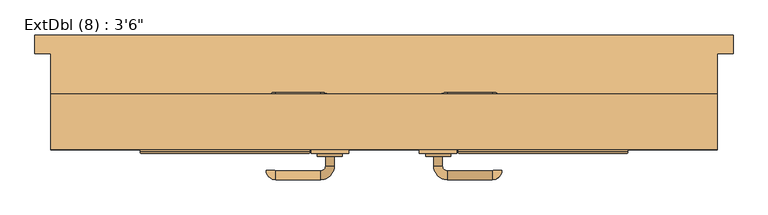
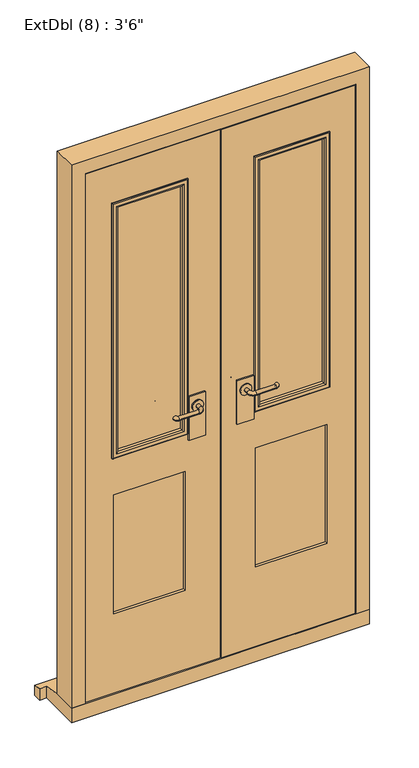
"""IFC4 building model written with IfcOpenShell, lengths in millimetres: door geometry."""

from ifc_helpers import new_model, si_unit, point, frame, frame_2d, origin, place, context, project, spatial, polyline, circle_curve, ellipse_curve, trimmed, segment, composite_curve, outline, extrude, faceted_brep, source, transform, mapped, element, save
from ifc_brep_helpers import plane_surface, cylinder_surface, revolved_surface, advanced_brep


def door_2576ec39(model_context):
    return source(origin(), model_context, "Body", "SolidModel", [
        extrude(outline(composite_curve([segment(trimmed(circle_curve(frame_2d((1050.0, 86.5)), 20.0), [point((1050.0, 66.5))], [point((1050.0, 106.5))], False, "CARTESIAN"), True, "CONTINUOUS"), segment(trimmed(circle_curve(frame_2d((1050.0, 86.5)), 20.0), [point((1050.0, 106.5))], [point((1050.0, 66.5))], False, "CARTESIAN"), True, "CONTINUOUS")], self_intersect=False)), frame((0.0, -88.3929895, 0.0), z_axis=(0.0, 1.0, 0.0), x_axis=(0.0, 0.0, 1.0)), (0.0, 0.0, 1.0), 4.5929895),
        advanced_brep(
        [(93.5, -88.3929895, 1050.0), (79.5, -88.3929895, 1050.0), (79.5, -103.8, 1050.0), (93.5, -103.8, 1050.0), (101.5, -125.8, 1050.0), (101.5, -111.8, 1050.0), (173.5, -125.8, 1050.0), (173.5, -111.8, 1050.0), (174.5, -110.8, 1050.0), (188.5, -110.8, 1050.0)],
        [
            (0, 1, circle_curve(frame((86.5, -88.3929895, 1050.0), z_axis=(0.0, 1.0, 0.0), x_axis=(-1.0, 0.0, 0.0)), 7.0)),
            (1, 0, circle_curve(frame((86.5, -88.3929895, 1050.0), z_axis=(0.0, 1.0, 0.0), x_axis=(-1.0, 0.0, 0.0)), 7.0)),
            (1, 2),
            (2, 3, circle_curve(frame((86.5, -103.8, 1050.0), z_axis=(0.0, 1.0, 0.0), x_axis=(-1.0, 0.0, 0.0)), 7.0)),
            (3, 0),
            (3, 2, circle_curve(frame((86.5, -103.8, 1050.0), z_axis=(0.0, 1.0, 0.0), x_axis=(-1.0, 0.0, 0.0)), 7.0)),
            (4, 5, circle_curve(frame((101.5, -118.8, 1050.0), z_axis=(-1.0, 0.0, 0.0), x_axis=(0.0, -1.0, 0.0)), 7.0)),
            (5, 3, circle_curve(frame((101.5, -103.8, 1050.0), z_axis=(0.0, 0.0, -1.0), x_axis=(-1.0, 0.0, 0.0)), 8.0)),
            (2, 4, circle_curve(frame((101.5, -103.8, 1050.0), z_axis=(0.0, 0.0, 1.0), x_axis=(-1.0, 0.0, 0.0)), 22.0)),
            (5, 4, circle_curve(frame((101.5, -118.8, 1050.0), z_axis=(-1.0, 0.0, 0.0), x_axis=(0.0, -1.0, 0.0)), 7.0)),
            (4, 6),
            (6, 7, circle_curve(frame((173.5, -118.8, 1050.0), z_axis=(-1.0, 0.0, 0.0), x_axis=(0.0, -1.0, 0.0)), 7.0)),
            (7, 5),
            (7, 6, circle_curve(frame((173.5, -118.8, 1050.0), z_axis=(-1.0, 0.0, 0.0), x_axis=(0.0, -1.0, 0.0)), 7.0)),
            (8, 9, circle_curve(frame((181.5, -110.8, 1050.0), z_axis=(0.0, 1.0, 0.0), x_axis=(1.0, 0.0, 0.0)), 7.0)),
            (9, 8, circle_curve(frame((181.5, -110.8, 1050.0), z_axis=(0.0, 1.0, 0.0), x_axis=(1.0, 0.0, 0.0)), 7.0)),
            (8, 7, circle_curve(frame((173.5, -110.8, 1050.0), z_axis=(0.0, 0.0, -1.0), x_axis=(0.0, -1.0, 0.0)), 1.0)),
            (6, 9, circle_curve(frame((173.5, -110.8, 1050.0), z_axis=(0.0, 0.0, 1.0), x_axis=(0.0, -1.0, 0.0)), 15.0)),
        ],
        [
            plane_surface(frame((86.5, -88.3929895, 1050.0), z_axis=(0.0, 1.0, 0.0), x_axis=(0.0, 0.0, 1.0))),
            cylinder_surface(frame((86.5, -88.3929895, 1050.0), z_axis=(0.0, 1.0, 0.0), x_axis=(-1.0, 0.0, 0.0)), 7.0),
            revolved_surface(trimmed(ellipse_curve(frame((86.5, -103.8, 1050.0), z_axis=(0.0, -1.0, 0.0), x_axis=(-1.0, 0.0, 0.0)), 7.0, 7.0), [point((93.5, -103.8, 1050.0))], [point((79.5, -103.8, 1050.0))], True, "CARTESIAN"), (101.5, -103.8, 1050.0), (0.0, 0.0, -1.0)),
            revolved_surface(trimmed(ellipse_curve(frame((86.5, -103.8, 1050.0), z_axis=(0.0, -1.0, 0.0), x_axis=(-1.0, 0.0, 0.0)), 7.0, 7.0), [point((79.5, -103.8, 1050.0))], [point((93.5, -103.8, 1050.0))], True, "CARTESIAN"), (101.5, -103.8, 1050.0), (0.0, 0.0, -1.0)),
            cylinder_surface(frame((101.5, -118.8, 1050.0), z_axis=(-1.0, 0.0, 0.0), x_axis=(0.0, -1.0, 0.0)), 7.0),
            plane_surface(frame((181.5, -110.8, 1050.0), z_axis=(0.0, 1.0, 0.0), x_axis=(0.0, 0.0, 1.0))),
            revolved_surface(trimmed(ellipse_curve(frame((173.5, -118.8, 1050.0), z_axis=(1.0, 0.0, 0.0), x_axis=(0.0, -1.0, 0.0)), 7.0, 7.0), [point((173.5, -111.8, 1050.0))], [point((173.5, -125.8, 1050.0))], True, "CARTESIAN"), (173.5, -110.8, 1050.0), (0.0, 0.0, -1.0)),
            revolved_surface(trimmed(ellipse_curve(frame((173.5, -118.8, 1050.0), z_axis=(1.0, 0.0, 0.0), x_axis=(0.0, -1.0, 0.0)), 7.0, 7.0), [point((173.5, -125.8, 1050.0))], [point((173.5, -111.8, 1050.0))], True, "CARTESIAN"), (173.5, -110.8, 1050.0), (0.0, 0.0, -1.0)),
        ],
        [
            (0, [[1, 2]]),
            (1, [[3, 4, 5, -2]]),
            (1, [[-5, 6, -3, -1]]),
            (2, [[7, 8, -4, 9]]),
            (3, [[10, -9, -6, -8]]),
            (4, [[11, 12, 13, -7]]),
            (4, [[-13, 14, -11, -10]]),
            (5, [[15, 16]]),
            (6, [[-15, 17, -12, 18]]),
            (7, [[-16, -18, -14, -17]]),
        ],
    ),
        extrude(outline(polyline([(116.5, -77.8), (116.5, -83.8), (56.5, -83.8), (56.5, -77.8), (116.5, -77.8)])), frame((0.0, 0.0, 925.0), z_axis=(0.0, 0.0, 1.0), x_axis=(1.0, 0.0, 0.0)), (0.0, 0.0, 1.0), 165.0),
        extrude(outline(composite_curve([segment(trimmed(circle_curve(frame_2d((1050.0, -86.5)), 20.0), [point((1050.0, -66.5))], [point((1050.0, -106.5))], False, "CARTESIAN"), True, "CONTINUOUS"), segment(trimmed(circle_curve(frame_2d((1050.0, -86.5)), 20.0), [point((1050.0, -106.5))], [point((1050.0, -66.5))], False, "CARTESIAN"), True, "CONTINUOUS")], self_intersect=False)), frame((0.0, -88.3929895, 0.0), z_axis=(0.0, 1.0, 0.0), x_axis=(0.0, 0.0, 1.0)), (0.0, 0.0, 1.0), 4.5929895),
        advanced_brep(
        [(-93.5, -88.3929895, 1050.0), (-79.5, -88.3929895, 1050.0), (-93.5, -103.8, 1050.0), (-79.5, -103.8, 1050.0), (-101.5, -125.8, 1050.0), (-101.5, -111.8, 1050.0), (-173.5, -111.8, 1050.0), (-173.5, -125.8, 1050.0), (-174.5, -110.8, 1050.0), (-188.5, -110.8, 1050.0)],
        [
            (0, 1, circle_curve(frame((-86.5, -88.3929895, 1050.0), z_axis=(0.0, 1.0, 0.0), x_axis=(1.0, 0.0, 0.0)), 7.0)),
            (1, 0, circle_curve(frame((-86.5, -88.3929895, 1050.0), z_axis=(0.0, 1.0, 0.0), x_axis=(1.0, 0.0, 0.0)), 7.0)),
            (0, 2),
            (2, 3, circle_curve(frame((-86.5, -103.8, 1050.0), z_axis=(0.0, 1.0, 0.0), x_axis=(1.0, 0.0, 0.0)), 7.0)),
            (3, 1),
            (3, 2, circle_curve(frame((-86.5, -103.8, 1050.0), z_axis=(0.0, 1.0, 0.0), x_axis=(1.0, 0.0, 0.0)), 7.0)),
            (4, 3, circle_curve(frame((-101.5, -103.8, 1050.0), z_axis=(0.0, 0.0, 1.0), x_axis=(1.0, 0.0, 0.0)), 22.0)),
            (2, 5, circle_curve(frame((-101.5, -103.8, 1050.0), z_axis=(0.0, 0.0, -1.0), x_axis=(1.0, 0.0, 0.0)), 8.0)),
            (5, 4, circle_curve(frame((-101.5, -118.8, 1050.0), z_axis=(1.0, 0.0, 0.0), x_axis=(0.0, -1.0, 0.0)), 7.0)),
            (4, 5, circle_curve(frame((-101.5, -118.8, 1050.0), z_axis=(1.0, 0.0, 0.0), x_axis=(0.0, -1.0, 0.0)), 7.0)),
            (5, 6),
            (6, 7, circle_curve(frame((-173.5, -118.8, 1050.0), z_axis=(1.0, 0.0, 0.0), x_axis=(0.0, -1.0, 0.0)), 7.0)),
            (7, 4),
            (7, 6, circle_curve(frame((-173.5, -118.8, 1050.0), z_axis=(1.0, 0.0, 0.0), x_axis=(0.0, -1.0, 0.0)), 7.0)),
            (8, 9, circle_curve(frame((-181.5, -110.8, 1050.0), z_axis=(0.0, 1.0, 0.0), x_axis=(-1.0, 0.0, 0.0)), 7.0)),
            (9, 8, circle_curve(frame((-181.5, -110.8, 1050.0), z_axis=(0.0, 1.0, 0.0), x_axis=(-1.0, 0.0, 0.0)), 7.0)),
            (9, 7, circle_curve(frame((-173.5, -110.8, 1050.0), z_axis=(0.0, 0.0, 1.0), x_axis=(0.0, -1.0, 0.0)), 15.0)),
            (6, 8, circle_curve(frame((-173.5, -110.8, 1050.0), z_axis=(0.0, 0.0, -1.0), x_axis=(0.0, -1.0, 0.0)), 1.0)),
        ],
        [
            plane_surface(frame((-86.5, -88.3929895, 1050.0), z_axis=(0.0, 1.0, 0.0), x_axis=(0.0, 0.0, 1.0))),
            cylinder_surface(frame((-86.5, -88.3929895, 1050.0), z_axis=(0.0, 1.0, 0.0), x_axis=(1.0, 0.0, 0.0)), 7.0),
            revolved_surface(trimmed(ellipse_curve(frame((-86.5, -103.8, 1050.0), z_axis=(0.0, 1.0, 0.0), x_axis=(1.0, 0.0, 0.0)), 7.0, 7.0), [point((-93.5, -103.8, 1050.0))], [point((-79.5, -103.8, 1050.0))], True, "CARTESIAN"), (-101.5, -103.8, 1050.0), (0.0, 0.0, -1.0)),
            revolved_surface(trimmed(ellipse_curve(frame((-86.5, -103.8, 1050.0), z_axis=(0.0, 1.0, 0.0), x_axis=(1.0, 0.0, 0.0)), 7.0, 7.0), [point((-79.5, -103.8, 1050.0))], [point((-93.5, -103.8, 1050.0))], True, "CARTESIAN"), (-101.5, -103.8, 1050.0), (0.0, 0.0, -1.0)),
            cylinder_surface(frame((-101.5, -118.8, 1050.0), z_axis=(1.0, 0.0, 0.0), x_axis=(0.0, -1.0, 0.0)), 7.0),
            plane_surface(frame((-181.5, -110.8, 1050.0), z_axis=(0.0, 1.0, 0.0), x_axis=(0.0, 0.0, 1.0))),
            revolved_surface(trimmed(ellipse_curve(frame((-173.5, -118.8, 1050.0), z_axis=(1.0, 0.0, 0.0), x_axis=(0.0, -1.0, 0.0)), 7.0, 7.0), [point((-173.5, -111.8, 1050.0))], [point((-173.5, -125.8, 1050.0))], True, "CARTESIAN"), (-173.5, -110.8, 1050.0), (0.0, 0.0, -1.0)),
            revolved_surface(trimmed(ellipse_curve(frame((-173.5, -118.8, 1050.0), z_axis=(1.0, 0.0, 0.0), x_axis=(0.0, -1.0, 0.0)), 7.0, 7.0), [point((-173.5, -125.8, 1050.0))], [point((-173.5, -111.8, 1050.0))], True, "CARTESIAN"), (-173.5, -110.8, 1050.0), (0.0, 0.0, -1.0)),
        ],
        [
            (0, [[1, 2]]),
            (1, [[-1, 3, 4, 5]]),
            (1, [[-2, -5, 6, -3]]),
            (2, [[7, -4, 8, 9]]),
            (3, [[-8, -6, -7, 10]]),
            (4, [[-9, 11, 12, 13]]),
            (4, [[-10, -13, 14, -11]]),
            (5, [[15, 16]]),
            (6, [[17, -12, 18, -16]]),
            (7, [[-18, -14, -17, -15]]),
        ],
    ),
        extrude(outline(polyline([(-116.5, -77.8), (-56.5, -77.8), (-56.5, -83.8), (-116.5, -83.8), (-116.5, -77.8)])), frame((0.0, 0.0, 925.0), z_axis=(0.0, 0.0, 1.0), x_axis=(1.0, 0.0, 0.0)), (0.0, 0.0, 1.0), 165.0),
        extrude(outline(composite_curve([segment(trimmed(circle_curve(frame_2d((1050.0, -86.5)), 20.0), [point((1050.0, -66.5))], [point((1050.0, -106.5))], False, "CARTESIAN"), True, "CONTINUOUS"), segment(trimmed(circle_curve(frame_2d((1050.0, -86.5)), 20.0), [point((1050.0, -106.5))], [point((1050.0, -66.5))], False, "CARTESIAN"), True, "CONTINUOUS")], self_intersect=False)), frame((0.0, -27.8, 0.0), z_axis=(0.0, 1.0, 0.0), x_axis=(0.0, 0.0, 1.0)), (0.0, 0.0, 1.0), 4.5929895),
        advanced_brep(
        [(-93.5, -23.2070105, 1050.0), (-79.5, -23.2070105, 1050.0), (-79.5, -7.8, 1050.0), (-93.5, -7.8, 1050.0), (-101.5, 14.2, 1050.0), (-101.5, 0.2, 1050.0), (-173.5, 14.2, 1050.0), (-173.5, 0.2, 1050.0), (-174.5, -0.8, 1050.0), (-188.5, -0.8, 1050.0)],
        [
            (0, 1, circle_curve(frame((-86.5, -23.2070105, 1050.0), z_axis=(0.0, -1.0, 0.0), x_axis=(1.0, 0.0, 0.0)), 7.0)),
            (1, 0, circle_curve(frame((-86.5, -23.2070105, 1050.0), z_axis=(0.0, -1.0, 0.0), x_axis=(1.0, 0.0, 0.0)), 7.0)),
            (1, 2),
            (2, 3, circle_curve(frame((-86.5, -7.8, 1050.0), z_axis=(0.0, -1.0, 0.0), x_axis=(1.0, 0.0, 0.0)), 7.0)),
            (3, 0),
            (3, 2, circle_curve(frame((-86.5, -7.8, 1050.0), z_axis=(0.0, -1.0, 0.0), x_axis=(1.0, 0.0, 0.0)), 7.0)),
            (4, 5, circle_curve(frame((-101.5, 7.2, 1050.0), z_axis=(1.0, 0.0, 0.0), x_axis=(0.0, 1.0, 0.0)), 7.0)),
            (5, 3, circle_curve(frame((-101.5, -7.8, 1050.0), z_axis=(0.0, 0.0, -1.0), x_axis=(1.0, 0.0, 0.0)), 8.0)),
            (2, 4, circle_curve(frame((-101.5, -7.8, 1050.0), z_axis=(0.0, 0.0, 1.0), x_axis=(1.0, 0.0, 0.0)), 22.0)),
            (5, 4, circle_curve(frame((-101.5, 7.2, 1050.0), z_axis=(1.0, 0.0, 0.0), x_axis=(0.0, 1.0, 0.0)), 7.0)),
            (4, 6),
            (6, 7, circle_curve(frame((-173.5, 7.2, 1050.0), z_axis=(1.0, 0.0, 0.0), x_axis=(0.0, 1.0, 0.0)), 7.0)),
            (7, 5),
            (7, 6, circle_curve(frame((-173.5, 7.2, 1050.0), z_axis=(1.0, 0.0, 0.0), x_axis=(0.0, 1.0, 0.0)), 7.0)),
            (8, 9, circle_curve(frame((-181.5, -0.8, 1050.0), z_axis=(0.0, -1.0, 0.0), x_axis=(-1.0, 0.0, 0.0)), 7.0)),
            (9, 8, circle_curve(frame((-181.5, -0.8, 1050.0), z_axis=(0.0, -1.0, 0.0), x_axis=(-1.0, 0.0, 0.0)), 7.0)),
            (8, 7, circle_curve(frame((-173.5, -0.8, 1050.0), z_axis=(0.0, 0.0, -1.0), x_axis=(0.0, 1.0, 0.0)), 1.0)),
            (6, 9, circle_curve(frame((-173.5, -0.8, 1050.0), z_axis=(0.0, 0.0, 1.0), x_axis=(0.0, 1.0, 0.0)), 15.0)),
        ],
        [
            plane_surface(frame((-86.5, -23.2070105, 1050.0), z_axis=(0.0, -1.0, 0.0), x_axis=(0.0, 0.0, 1.0))),
            cylinder_surface(frame((-86.5, -23.2070105, 1050.0), z_axis=(0.0, -1.0, 0.0), x_axis=(1.0, 0.0, 0.0)), 7.0),
            revolved_surface(trimmed(ellipse_curve(frame((-86.5, -7.8, 1050.0), z_axis=(0.0, 1.0, 0.0), x_axis=(1.0, 0.0, 0.0)), 7.0, 7.0), [point((-93.5, -7.8, 1050.0))], [point((-79.5, -7.8, 1050.0))], True, "CARTESIAN"), (-101.5, -7.8, 1050.0), (0.0, 0.0, -1.0)),
            revolved_surface(trimmed(ellipse_curve(frame((-86.5, -7.8, 1050.0), z_axis=(0.0, 1.0, 0.0), x_axis=(1.0, 0.0, 0.0)), 7.0, 7.0), [point((-79.5, -7.8, 1050.0))], [point((-93.5, -7.8, 1050.0))], True, "CARTESIAN"), (-101.5, -7.8, 1050.0), (0.0, 0.0, -1.0)),
            cylinder_surface(frame((-101.5, 7.2, 1050.0), z_axis=(1.0, 0.0, 0.0), x_axis=(0.0, 1.0, 0.0)), 7.0),
            plane_surface(frame((-181.5, -0.8, 1050.0), z_axis=(0.0, -1.0, 0.0), x_axis=(0.0, 0.0, 1.0))),
            revolved_surface(trimmed(ellipse_curve(frame((-173.5, 7.2, 1050.0), z_axis=(-1.0, 0.0, 0.0), x_axis=(0.0, 1.0, 0.0)), 7.0, 7.0), [point((-173.5, 0.2, 1050.0))], [point((-173.5, 14.2, 1050.0))], True, "CARTESIAN"), (-173.5, -0.8, 1050.0), (0.0, 0.0, -1.0)),
            revolved_surface(trimmed(ellipse_curve(frame((-173.5, 7.2, 1050.0), z_axis=(-1.0, 0.0, 0.0), x_axis=(0.0, 1.0, 0.0)), 7.0, 7.0), [point((-173.5, 14.2, 1050.0))], [point((-173.5, 0.2, 1050.0))], True, "CARTESIAN"), (-173.5, -0.8, 1050.0), (0.0, 0.0, -1.0)),
        ],
        [
            (0, [[1, 2]]),
            (1, [[3, 4, 5, -2]]),
            (1, [[-5, 6, -3, -1]]),
            (2, [[7, 8, -4, 9]]),
            (3, [[10, -9, -6, -8]]),
            (4, [[11, 12, 13, -7]]),
            (4, [[-13, 14, -11, -10]]),
            (5, [[15, 16]]),
            (6, [[-15, 17, -12, 18]]),
            (7, [[-16, -18, -14, -17]]),
        ],
    ),
        extrude(outline(polyline([(-116.5, -33.8), (-116.5, -27.8), (-56.5, -27.8), (-56.5, -33.8), (-116.5, -33.8)])), frame((0.0, 0.0, 925.0), z_axis=(0.0, 0.0, 1.0), x_axis=(1.0, 0.0, 0.0)), (0.0, 0.0, 1.0), 165.0),
        extrude(outline(composite_curve([segment(trimmed(circle_curve(frame_2d((1050.0, 86.5)), 20.0), [point((1050.0, 66.5))], [point((1050.0, 106.5))], False, "CARTESIAN"), True, "CONTINUOUS"), segment(trimmed(circle_curve(frame_2d((1050.0, 86.5)), 20.0), [point((1050.0, 106.5))], [point((1050.0, 66.5))], False, "CARTESIAN"), True, "CONTINUOUS")], self_intersect=False)), frame((0.0, -27.8, 0.0), z_axis=(0.0, 1.0, 0.0), x_axis=(0.0, 0.0, 1.0)), (0.0, 0.0, 1.0), 4.5929895),
        advanced_brep(
        [(93.5, -23.2070105, 1050.0), (79.5, -23.2070105, 1050.0), (93.5, -7.8, 1050.0), (79.5, -7.8, 1050.0), (101.5, 14.2, 1050.0), (101.5, 0.2, 1050.0), (173.5, 0.2, 1050.0), (173.5, 14.2, 1050.0), (174.5, -0.8, 1050.0), (188.5, -0.8, 1050.0)],
        [
            (0, 1, circle_curve(frame((86.5, -23.2070105, 1050.0), z_axis=(0.0, -1.0, 0.0), x_axis=(-1.0, 0.0, 0.0)), 7.0)),
            (1, 0, circle_curve(frame((86.5, -23.2070105, 1050.0), z_axis=(0.0, -1.0, 0.0), x_axis=(-1.0, 0.0, 0.0)), 7.0)),
            (0, 2),
            (2, 3, circle_curve(frame((86.5, -7.8, 1050.0), z_axis=(0.0, -1.0, 0.0), x_axis=(-1.0, 0.0, 0.0)), 7.0)),
            (3, 1),
            (3, 2, circle_curve(frame((86.5, -7.8, 1050.0), z_axis=(0.0, -1.0, 0.0), x_axis=(-1.0, 0.0, 0.0)), 7.0)),
            (4, 3, circle_curve(frame((101.5, -7.8, 1050.0), z_axis=(0.0, 0.0, 1.0), x_axis=(-1.0, 0.0, 0.0)), 22.0)),
            (2, 5, circle_curve(frame((101.5, -7.8, 1050.0), z_axis=(0.0, 0.0, -1.0), x_axis=(-1.0, 0.0, 0.0)), 8.0)),
            (5, 4, circle_curve(frame((101.5, 7.2, 1050.0), z_axis=(-1.0, 0.0, 0.0), x_axis=(0.0, 1.0, 0.0)), 7.0)),
            (4, 5, circle_curve(frame((101.5, 7.2, 1050.0), z_axis=(-1.0, 0.0, 0.0), x_axis=(0.0, 1.0, 0.0)), 7.0)),
            (5, 6),
            (6, 7, circle_curve(frame((173.5, 7.2, 1050.0), z_axis=(-1.0, 0.0, 0.0), x_axis=(0.0, 1.0, 0.0)), 7.0)),
            (7, 4),
            (7, 6, circle_curve(frame((173.5, 7.2, 1050.0), z_axis=(-1.0, 0.0, 0.0), x_axis=(0.0, 1.0, 0.0)), 7.0)),
            (8, 9, circle_curve(frame((181.5, -0.8, 1050.0), z_axis=(0.0, -1.0, 0.0), x_axis=(1.0, 0.0, 0.0)), 7.0)),
            (9, 8, circle_curve(frame((181.5, -0.8, 1050.0), z_axis=(0.0, -1.0, 0.0), x_axis=(1.0, 0.0, 0.0)), 7.0)),
            (9, 7, circle_curve(frame((173.5, -0.8, 1050.0), z_axis=(0.0, 0.0, 1.0), x_axis=(0.0, 1.0, 0.0)), 15.0)),
            (6, 8, circle_curve(frame((173.5, -0.8, 1050.0), z_axis=(0.0, 0.0, -1.0), x_axis=(0.0, 1.0, 0.0)), 1.0)),
        ],
        [
            plane_surface(frame((86.5, -23.2070105, 1050.0), z_axis=(0.0, -1.0, 0.0), x_axis=(0.0, 0.0, 1.0))),
            cylinder_surface(frame((86.5, -23.2070105, 1050.0), z_axis=(0.0, -1.0, 0.0), x_axis=(-1.0, 0.0, 0.0)), 7.0),
            revolved_surface(trimmed(ellipse_curve(frame((86.5, -7.8, 1050.0), z_axis=(0.0, -1.0, 0.0), x_axis=(-1.0, 0.0, 0.0)), 7.0, 7.0), [point((93.5, -7.8, 1050.0))], [point((79.5, -7.8, 1050.0))], True, "CARTESIAN"), (101.5, -7.8, 1050.0), (0.0, 0.0, -1.0)),
            revolved_surface(trimmed(ellipse_curve(frame((86.5, -7.8, 1050.0), z_axis=(0.0, -1.0, 0.0), x_axis=(-1.0, 0.0, 0.0)), 7.0, 7.0), [point((79.5, -7.8, 1050.0))], [point((93.5, -7.8, 1050.0))], True, "CARTESIAN"), (101.5, -7.8, 1050.0), (0.0, 0.0, -1.0)),
            cylinder_surface(frame((101.5, 7.2, 1050.0), z_axis=(-1.0, 0.0, 0.0), x_axis=(0.0, 1.0, 0.0)), 7.0),
            plane_surface(frame((181.5, -0.8, 1050.0), z_axis=(0.0, -1.0, 0.0), x_axis=(0.0, 0.0, 1.0))),
            revolved_surface(trimmed(ellipse_curve(frame((173.5, 7.2, 1050.0), z_axis=(-1.0, 0.0, 0.0), x_axis=(0.0, 1.0, 0.0)), 7.0, 7.0), [point((173.5, 0.2, 1050.0))], [point((173.5, 14.2, 1050.0))], True, "CARTESIAN"), (173.5, -0.8, 1050.0), (0.0, 0.0, -1.0)),
            revolved_surface(trimmed(ellipse_curve(frame((173.5, 7.2, 1050.0), z_axis=(-1.0, 0.0, 0.0), x_axis=(0.0, 1.0, 0.0)), 7.0, 7.0), [point((173.5, 14.2, 1050.0))], [point((173.5, 0.2, 1050.0))], True, "CARTESIAN"), (173.5, -0.8, 1050.0), (0.0, 0.0, -1.0)),
        ],
        [
            (0, [[1, 2]]),
            (1, [[-1, 3, 4, 5]]),
            (1, [[-2, -5, 6, -3]]),
            (2, [[7, -4, 8, 9]]),
            (3, [[-8, -6, -7, 10]]),
            (4, [[-9, 11, 12, 13]]),
            (4, [[-10, -13, 14, -11]]),
            (5, [[15, 16]]),
            (6, [[17, -12, 18, -16]]),
            (7, [[-18, -14, -17, -15]]),
        ],
    ),
        extrude(outline(polyline([(116.5, -33.8), (56.5, -33.8), (56.5, -27.8), (116.5, -27.8), (116.5, -33.8)])), frame((0.0, 0.0, 925.0), z_axis=(0.0, 0.0, 1.0), x_axis=(1.0, 0.0, 0.0)), (0.0, 0.0, 1.0), 165.0),
        faceted_brep([(462.9, 11.2, 54.5), (533.4, 11.2, 54.5), (533.4, -77.8, 54.5), (484.9, -77.8, 54.5), (484.9, -30.8, 54.5), (462.9, -30.8, 54.5), (462.9, 11.2, 2039.5), (-462.9, 11.2, 2039.5), (-462.9, 11.2, 54.5), (-533.4, 11.2, 54.5), (-533.4, 11.2, 2110.0), (533.4, 11.2, 2110.0), (533.4, -77.8, 2110.0), (-533.4, -77.8, 2110.0), (-533.4, -77.8, 54.5), (-484.9, -77.8, 54.5), (-484.9, -77.8, 2061.5), (484.9, -77.8, 2061.5), (484.9, -30.8, 2061.5), (-484.9, -30.8, 2061.5), (-484.9, -30.8, 54.5), (-462.9, -30.8, 54.5), (-462.9, -30.8, 2039.5), (462.9, -30.8, 2039.5)], [[[0, 1, 2, 3, 4, 5]], [[1, 0, 6, 7, 8, 9, 10, 11]], [[2, 1, 11, 12]], [[3, 2, 12, 13, 14, 15, 16, 17]], [[4, 3, 17, 18]], [[5, 4, 18, 19, 20, 21, 22, 23]], [[0, 5, 23, 6]], [[7, 22, 21, 8]], [[8, 21, 20, 15, 14, 9]], [[13, 10, 9, 14]], [[19, 16, 15, 20]], [[12, 11, 10, 13]], [[18, 17, 16, 19]], [[6, 23, 22, 7]]]),
        extrude(outline(polyline([(58.5, 481.9), (2058.5, 481.9), (2058.5, 1.5), (58.5, 1.5), (58.5, 481.9)]), holes=[polyline([(1908.5, 381.9), (958.5, 381.9), (958.5, 126.5), (1908.5, 126.5), (1908.5, 381.9)]), polyline([(808.5, 126.5), (808.5, 381.9), (358.5, 381.9), (358.5, 126.5), (808.5, 126.5)])]), frame((0.0, -77.8, 0.0), z_axis=(0.0, 1.0, 0.0), x_axis=(0.0, 0.0, 1.0)), (0.0, 0.0, 1.0), 44.0),
        extrude(outline(polyline([(58.5, -481.9), (58.5, -1.5), (2058.5, -1.5), (2058.5, -481.9), (58.5, -481.9)]), holes=[polyline([(1908.5, -126.5), (958.5, -126.5), (958.5, -381.9), (1908.5, -381.9), (1908.5, -126.5)]), polyline([(808.5, -381.9), (808.5, -126.5), (358.5, -126.5), (358.5, -381.9), (808.5, -381.9)])]), frame((0.0, -77.8, 0.0), z_axis=(0.0, 1.0, 0.0), x_axis=(0.0, 0.0, 1.0)), (0.0, 0.0, 1.0), 44.0),
        faceted_brep([(558.4, 106.2, 0.0), (558.4, 106.2, 38.5947221), (558.4, 76.2, 43.6174415), (558.4, 76.2, 0.0), (-558.4, 106.2, 38.5947221), (-558.4, 106.2, 0.0), (-558.4, 76.2, 0.0), (-558.4, 76.2, 43.6174415), (533.4, 76.2, 0.0), (533.4, -77.8, 0.0), (-533.4, -77.8, 0.0), (-533.4, 76.2, 0.0), (-533.4, 76.2, 43.6174415), (-533.4, 11.2, 54.5), (533.4, 11.2, 54.5), (533.4, 76.2, 43.6174415), (-533.4, -77.8, 54.5), (533.4, -77.8, 54.5)], [[[0, 1, 2, 3]], [[4, 5, 6, 7]], [[5, 0, 3, 8, 9, 10, 11, 6]], [[1, 0, 5, 4]], [[1, 4, 7, 12, 13, 14, 15, 2]], [[13, 16, 17, 14]], [[16, 10, 9, 17]], [[12, 11, 10, 16, 13]], [[11, 12, 7, 6]], [[8, 15, 14, 17, 9]], [[15, 8, 3, 2]]]),
        extrude(outline(polyline([(126.5, -43.8), (380.3390207, -43.8), (380.3390207, -67.8), (126.5, -67.8), (126.5, -43.8)])), frame((0.0, 0.0, 958.5), z_axis=(0.0, 0.0, 1.0), x_axis=(1.0, 0.0, 0.0)), (0.0, 0.0, 1.0), 950.0),
        extrude(outline(polyline([(-381.9, -43.8), (-126.5, -43.8), (-126.5, -67.8), (-381.9, -67.8), (-381.9, -43.8)])), frame((0.0, 0.0, 958.5), z_axis=(0.0, 0.0, 1.0), x_axis=(1.0, 0.0, 0.0)), (0.0, 0.0, 1.0), 950.0),
        extrude(outline(polyline([(381.9, -67.8), (126.5, -67.8), (126.5, -43.8), (381.9, -43.8), (381.9, -67.8)])), frame((0.0, 0.0, 358.5), z_axis=(0.0, 0.0, 1.0), x_axis=(1.0, 0.0, 0.0)), (0.0, 0.0, 1.0), 450.0),
        extrude(outline(polyline([(-126.5, -67.8), (-381.9, -67.8), (-381.9, -43.8), (-126.5, -43.8), (-126.5, -67.8)])), frame((0.0, 0.0, 358.5), z_axis=(0.0, 0.0, 1.0), x_axis=(1.0, 0.0, 0.0)), (0.0, 0.0, 1.0), 450.0),
        advanced_brep(
        [(118.5, -29.8, 950.5), (118.5, -33.8, 950.5), (118.5, -33.8, 1916.5), (118.5, -29.8, 1916.5), (120.5, -27.8, 952.5), (120.5, -27.8, 1914.5), (138.5, -32.8, 970.5), (133.5, -27.8, 965.5), (133.5, -27.8, 1901.5), (138.5, -32.8, 1896.5), (138.5, -43.8, 970.5), (138.5, -43.8, 1896.5), (126.5, -33.8, 958.5), (126.5, -43.8, 958.5), (126.5, -43.8, 1908.5), (126.5, -33.8, 1908.5), (389.9, -33.8, 1916.5), (389.9, -29.8, 1916.5), (387.9, -27.8, 1914.5), (374.9, -27.8, 1901.5), (369.9, -32.8, 1896.5), (369.9, -43.8, 1896.5), (381.9, -43.8, 1908.5), (381.9, -33.8, 1908.5), (389.9, -33.8, 950.5), (389.9, -29.8, 950.5), (387.9, -27.8, 952.5), (374.9, -27.8, 965.5), (369.9, -32.8, 970.5), (369.9, -43.8, 970.5), (381.9, -43.8, 958.5), (381.9, -33.8, 958.5)],
        [
            (0, 1),
            (1, 2),
            (2, 3),
            (3, 0),
            (4, 0, ellipse_curve(frame((120.5, -29.8, 952.5), z_axis=(-0.7071067811865474, 0.0, 0.7071067811865476), x_axis=(-0.7071067811865475, 0.0, -0.7071067811865476)), 2.8284271, 2.0)),
            (3, 5, ellipse_curve(frame((120.5, -29.8, 1914.5), z_axis=(-0.7071067811865476, 0.0, -0.7071067811865474), x_axis=(0.7071067811865474, 0.0, -0.7071067811865477)), 2.8284271, 2.0)),
            (5, 4),
            (6, 7, ellipse_curve(frame((133.5, -32.8, 965.5), z_axis=(-0.7071067811865474, 0.0, 0.7071067811865476), x_axis=(-0.7071067811865475, 0.0, -0.7071067811865476)), 7.0710678, 5.0)),
            (7, 8),
            (8, 9, ellipse_curve(frame((133.5, -32.8, 1901.5), z_axis=(-0.7071067811865476, 0.0, -0.7071067811865474), x_axis=(0.7071067811865474, 0.0, -0.7071067811865477)), 7.0710678, 5.0)),
            (9, 6),
            (10, 6),
            (9, 11),
            (11, 10),
            (12, 13),
            (13, 14),
            (14, 15),
            (15, 12),
            (2, 16),
            (16, 17),
            (17, 3),
            (17, 18, ellipse_curve(frame((387.9, -29.8, 1914.5), z_axis=(-0.7071067811865472, 0.0, 0.7071067811865477), x_axis=(-0.7071067811865479, 0.0, -0.7071067811865471)), 2.8284271, 2.0)),
            (18, 5),
            (8, 19),
            (19, 20, ellipse_curve(frame((374.9, -32.8, 1901.5), z_axis=(-0.7071067811865472, 0.0, 0.7071067811865477), x_axis=(-0.7071067811865479, 0.0, -0.7071067811865471)), 7.0710678, 5.0)),
            (20, 9),
            (20, 21),
            (21, 11),
            (14, 22),
            (22, 23),
            (23, 15),
            (16, 24),
            (24, 25),
            (25, 17),
            (25, 26, ellipse_curve(frame((387.9, -29.8, 952.5), z_axis=(0.7071067811865478, 0.0, 0.7071067811865472), x_axis=(-0.7071067811865471, 0.0, 0.7071067811865478)), 2.8284271, 2.0)),
            (26, 18),
            (19, 27),
            (27, 28, ellipse_curve(frame((374.9, -32.8, 965.5), z_axis=(0.7071067811865478, 0.0, 0.7071067811865472), x_axis=(-0.7071067811865471, 0.0, 0.7071067811865478)), 7.0710678, 5.0)),
            (28, 20),
            (28, 29),
            (29, 21),
            (22, 30),
            (30, 31),
            (31, 23),
            (24, 1),
            (0, 25),
            (4, 26),
            (7, 27),
            (6, 28),
            (10, 29),
            (13, 30),
            (12, 31),
        ],
        [
            plane_surface(frame((118.5, -33.8, 950.5), z_axis=(-1.0, 0.0, 0.0), x_axis=(0.0, 0.0, 1.0))),
            cylinder_surface(frame((120.5, -29.8, 958.5), z_axis=(0.0, 0.0, -1.0), x_axis=(-1.0, 0.0, 0.0)), 2.0),
            cylinder_surface(frame((133.5, -32.8, 958.5), z_axis=(0.0, 0.0, -1.0), x_axis=(-1.0, 0.0, 0.0)), 5.0),
            plane_surface(frame((138.5, -32.8, 970.5), z_axis=(1.0, 0.0, 0.0), x_axis=(0.0, 0.0, 1.0))),
            plane_surface(frame((126.5, -43.8, 958.5), z_axis=(-1.0, 0.0, 0.0), x_axis=(0.0, 0.0, 1.0))),
            plane_surface(frame((118.5, -33.8, 1916.5), z_axis=(0.0, 0.0, 1.0), x_axis=(1.0, 0.0, 0.0))),
            cylinder_surface(frame((126.5, -29.8, 1914.5), z_axis=(-1.0, 0.0, 0.0), x_axis=(0.0, 0.0, 1.0)), 2.0),
            cylinder_surface(frame((126.5, -32.8, 1901.5), z_axis=(-1.0, 0.0, 0.0), x_axis=(0.0, 0.0, 1.0)), 5.0),
            plane_surface(frame((138.5, -32.8, 1896.5), z_axis=(0.0, 0.0, -1.0), x_axis=(1.0, 0.0, 0.0))),
            plane_surface(frame((126.5, -43.8, 1908.5), z_axis=(0.0, 0.0, 1.0), x_axis=(1.0, 0.0, 0.0))),
            plane_surface(frame((389.9, -33.8, 1916.5), z_axis=(1.0, 0.0, 0.0), x_axis=(0.0, 0.0, -1.0))),
            cylinder_surface(frame((387.9, -29.8, 1908.5), z_axis=(0.0, 0.0, 1.0), x_axis=(1.0, 0.0, 0.0)), 2.0),
            cylinder_surface(frame((374.9, -32.8, 1908.5), z_axis=(0.0, 0.0, 1.0), x_axis=(1.0, 0.0, 0.0)), 5.0),
            plane_surface(frame((369.9, -32.8, 1896.5), z_axis=(-1.0, 0.0, 0.0), x_axis=(0.0, 0.0, -1.0))),
            plane_surface(frame((381.9, -43.8, 1908.5), z_axis=(1.0, 0.0, 0.0), x_axis=(0.0, 0.0, -1.0))),
            plane_surface(frame((389.9, -33.8, 950.5), z_axis=(0.0, 0.0, -1.0), x_axis=(-1.0, 0.0, 0.0))),
            cylinder_surface(frame((381.9, -29.8, 952.5), z_axis=(1.0, 0.0, 0.0), x_axis=(0.0, 0.0, -1.0)), 2.0),
            plane_surface(frame((387.9, -27.8, 952.5), z_axis=(0.0, 1.0, 0.0), x_axis=(-1.0, 0.0, 0.0))),
            cylinder_surface(frame((381.9, -32.8, 965.5), z_axis=(1.0, 0.0, 0.0), x_axis=(0.0, 0.0, -1.0)), 5.0),
            plane_surface(frame((369.9, -32.8, 970.5), z_axis=(0.0, 0.0, 1.0), x_axis=(-1.0, 0.0, 0.0))),
            plane_surface(frame((369.9, -43.8, 970.5), z_axis=(0.0, -1.0, 0.0), x_axis=(-1.0, 0.0, 0.0))),
            plane_surface(frame((381.9, -43.8, 958.5), z_axis=(0.0, 0.0, -1.0), x_axis=(-1.0, 0.0, 0.0))),
            plane_surface(frame((381.9, -33.8, 958.5), z_axis=(0.0, -1.0, 0.0), x_axis=(-1.0, 0.0, 0.0))),
        ],
        [
            (0, [[1, 2, 3, 4]]),
            (1, [[5, -4, 6, 7]]),
            (2, [[8, 9, 10, 11]]),
            (3, [[12, -11, 13, 14]]),
            (4, [[15, 16, 17, 18]]),
            (5, [[-3, 19, 20, 21]]),
            (6, [[-6, -21, 22, 23]]),
            (7, [[-10, 24, 25, 26]]),
            (8, [[-13, -26, 27, 28]]),
            (9, [[-17, 29, 30, 31]]),
            (10, [[-20, 32, 33, 34]]),
            (11, [[-22, -34, 35, 36]]),
            (12, [[-25, 37, 38, 39]]),
            (13, [[-27, -39, 40, 41]]),
            (14, [[-30, 42, 43, 44]]),
            (15, [[-33, 45, -1, 46]]),
            (16, [[-35, -46, -5, 47]]),
            (17, [[-23, -36, -47, -7], [48, -37, -24, -9]]),
            (18, [[-38, -48, -8, 49]]),
            (19, [[-40, -49, -12, 50]]),
            (20, [[51, -42, -29, -16], [-28, -41, -50, -14]]),
            (21, [[-43, -51, -15, 52]]),
            (22, [[-45, -32, -19, -2], [-31, -44, -52, -18]]),
        ],
    ),
        advanced_brep(
        [(381.9, -67.8, 1908.5), (381.9, -77.8, 1908.5), (381.9, -77.8, 958.5), (381.9, -67.8, 958.5), (369.9, -78.8, 1896.5), (369.9, -67.8, 1896.5), (369.9, -67.8, 970.5), (369.9, -78.8, 970.5), (374.9, -83.8, 1901.5), (374.9, -83.8, 965.5), (389.9, -81.8, 1916.5), (387.9, -83.8, 1914.5), (387.9, -83.8, 952.5), (389.9, -81.8, 950.5), (389.9, -77.8, 1916.5), (389.9, -77.8, 950.5), (126.5, -77.8, 958.5), (126.5, -67.8, 958.5), (138.5, -67.8, 970.5), (138.5, -78.8, 970.5), (133.5, -83.8, 965.5), (120.5, -83.8, 952.5), (118.5, -81.8, 950.5), (118.5, -77.8, 950.5), (126.5, -77.8, 1908.5), (126.5, -67.8, 1908.5), (138.5, -67.8, 1896.5), (138.5, -78.8, 1896.5), (133.5, -83.8, 1901.5), (120.5, -83.8, 1914.5), (118.5, -81.8, 1916.5), (118.5, -77.8, 1916.5)],
        [
            (0, 1),
            (1, 2),
            (2, 3),
            (3, 0),
            (4, 5),
            (5, 6),
            (6, 7),
            (7, 4),
            (8, 4, ellipse_curve(frame((374.9, -78.8, 1901.5), z_axis=(0.707106781186552, 0.0, -0.707106781186543), x_axis=(0.707106781186543, 0.0, 0.707106781186552)), 7.0710678, 5.0)),
            (7, 9, ellipse_curve(frame((374.9, -78.8, 965.5), z_axis=(0.7071067811865429, 0.0, 0.707106781186552), x_axis=(-0.7071067811865519, 0.0, 0.707106781186543)), 7.0710678, 5.0)),
            (9, 8),
            (10, 11, ellipse_curve(frame((387.9, -81.8, 1914.5), z_axis=(0.707106781186552, 0.0, -0.707106781186543), x_axis=(0.707106781186543, 0.0, 0.707106781186552)), 2.8284271, 2.0)),
            (11, 12),
            (12, 13, ellipse_curve(frame((387.9, -81.8, 952.5), z_axis=(0.7071067811865429, 0.0, 0.707106781186552), x_axis=(-0.7071067811865519, 0.0, 0.707106781186543)), 2.8284271, 2.0)),
            (13, 10),
            (14, 10),
            (13, 15),
            (15, 14),
            (2, 16),
            (16, 17),
            (17, 3),
            (6, 18),
            (18, 19),
            (19, 7),
            (19, 20, ellipse_curve(frame((133.5, -78.8, 965.5), z_axis=(0.707106781186552, 0.0, -0.707106781186543), x_axis=(0.707106781186543, 0.0, 0.707106781186552)), 7.0710678, 5.0)),
            (20, 9),
            (12, 21),
            (21, 22, ellipse_curve(frame((120.5, -81.8, 952.5), z_axis=(0.707106781186552, 0.0, -0.707106781186543), x_axis=(0.707106781186543, 0.0, 0.707106781186552)), 2.8284271, 2.0)),
            (22, 13),
            (22, 23),
            (23, 15),
            (16, 24),
            (24, 25),
            (25, 17),
            (18, 26),
            (26, 27),
            (27, 19),
            (27, 28, ellipse_curve(frame((133.5, -78.8, 1901.5), z_axis=(-0.7071067811865431, 0.0, -0.707106781186552), x_axis=(0.707106781186552, 0.0, -0.7071067811865429)), 7.0710678, 5.0)),
            (28, 20),
            (21, 29),
            (29, 30, ellipse_curve(frame((120.5, -81.8, 1914.5), z_axis=(-0.7071067811865431, 0.0, -0.707106781186552), x_axis=(0.707106781186552, 0.0, -0.7071067811865429)), 2.8284271, 2.0)),
            (30, 22),
            (30, 31),
            (31, 23),
            (31, 14),
            (1, 24),
            (0, 25),
            (5, 26),
            (4, 27),
            (8, 28),
            (11, 29),
            (10, 30),
        ],
        [
            plane_surface(frame((381.9, -77.8, 1908.5), z_axis=(1.0, 0.0, 0.0), x_axis=(0.0, 0.0, -1.0))),
            plane_surface(frame((369.9, -67.8, 1896.5), z_axis=(-1.0, 0.0, 0.0), x_axis=(0.0, 0.0, -1.0))),
            cylinder_surface(frame((374.9, -78.8, 1908.5), z_axis=(0.0, 0.0, 1.0), x_axis=(1.0, 0.0, 0.0)), 5.0),
            cylinder_surface(frame((387.9, -81.8, 1908.5), z_axis=(0.0, 0.0, 1.0), x_axis=(1.0, 0.0, 0.0)), 2.0),
            plane_surface(frame((389.9, -81.8, 1916.5), z_axis=(1.0, 0.0, 0.0), x_axis=(0.0, 0.0, -1.0))),
            plane_surface(frame((381.9, -77.8, 958.5), z_axis=(0.0, 0.0, -1.0), x_axis=(-1.0, 0.0, 0.0))),
            plane_surface(frame((369.9, -67.8, 970.5), z_axis=(0.0, 0.0, 1.0), x_axis=(-1.0, 0.0, 0.0))),
            cylinder_surface(frame((381.9, -78.8, 965.5), z_axis=(1.0, 0.0, 0.0), x_axis=(0.0, 0.0, -1.0)), 5.0),
            cylinder_surface(frame((381.9, -81.8, 952.5), z_axis=(1.0, 0.0, 0.0), x_axis=(0.0, 0.0, -1.0)), 2.0),
            plane_surface(frame((389.9, -81.8, 950.5), z_axis=(0.0, 0.0, -1.0), x_axis=(-1.0, 0.0, 0.0))),
            plane_surface(frame((126.5, -77.8, 958.5), z_axis=(-1.0, 0.0, 0.0), x_axis=(0.0, 0.0, 1.0))),
            plane_surface(frame((138.5, -67.8, 970.5), z_axis=(1.0, 0.0, 0.0), x_axis=(0.0, 0.0, 1.0))),
            cylinder_surface(frame((133.5, -78.8, 958.5), z_axis=(0.0, 0.0, -1.0), x_axis=(-1.0, 0.0, 0.0)), 5.0),
            cylinder_surface(frame((120.5, -81.8, 958.5), z_axis=(0.0, 0.0, -1.0), x_axis=(-1.0, 0.0, 0.0)), 2.0),
            plane_surface(frame((118.5, -81.8, 950.5), z_axis=(-1.0, 0.0, 0.0), x_axis=(0.0, 0.0, 1.0))),
            plane_surface(frame((118.5, -77.8, 1916.5), z_axis=(0.0, 1.0, 0.0), x_axis=(1.0, 0.0, 0.0))),
            plane_surface(frame((126.5, -77.8, 1908.5), z_axis=(0.0, 0.0, 1.0), x_axis=(1.0, 0.0, 0.0))),
            plane_surface(frame((126.5, -67.8, 1908.5), z_axis=(0.0, 1.0, 0.0), x_axis=(1.0, 0.0, 0.0))),
            plane_surface(frame((138.5, -67.8, 1896.5), z_axis=(0.0, 0.0, -1.0), x_axis=(1.0, 0.0, 0.0))),
            cylinder_surface(frame((126.5, -78.8, 1901.5), z_axis=(-1.0, 0.0, 0.0), x_axis=(0.0, 0.0, 1.0)), 5.0),
            plane_surface(frame((133.5, -83.8, 1901.5), z_axis=(0.0, -1.0, 0.0), x_axis=(1.0, 0.0, 0.0))),
            cylinder_surface(frame((126.5, -81.8, 1914.5), z_axis=(-1.0, 0.0, 0.0), x_axis=(0.0, 0.0, 1.0)), 2.0),
            plane_surface(frame((118.5, -81.8, 1916.5), z_axis=(0.0, 0.0, 1.0), x_axis=(1.0, 0.0, 0.0))),
        ],
        [
            (0, [[1, 2, 3, 4]]),
            (1, [[5, 6, 7, 8]]),
            (2, [[9, -8, 10, 11]]),
            (3, [[12, 13, 14, 15]]),
            (4, [[16, -15, 17, 18]]),
            (5, [[-3, 19, 20, 21]]),
            (6, [[-7, 22, 23, 24]]),
            (7, [[-10, -24, 25, 26]]),
            (8, [[-14, 27, 28, 29]]),
            (9, [[-17, -29, 30, 31]]),
            (10, [[-20, 32, 33, 34]]),
            (11, [[-23, 35, 36, 37]]),
            (12, [[-25, -37, 38, 39]]),
            (13, [[-28, 40, 41, 42]]),
            (14, [[-30, -42, 43, 44]]),
            (15, [[-31, -44, 45, -18], [46, -32, -19, -2]]),
            (16, [[-33, -46, -1, 47]]),
            (17, [[-21, -34, -47, -4], [48, -35, -22, -6]]),
            (18, [[-36, -48, -5, 49]]),
            (19, [[-38, -49, -9, 50]]),
            (20, [[51, -40, -27, -13], [-26, -39, -50, -11]]),
            (21, [[-41, -51, -12, 52]]),
            (22, [[-43, -52, -16, -45]]),
        ],
    ),
        advanced_brep(
        [(-126.5, -67.8, 1908.5), (-126.5, -77.8, 1908.5), (-126.5, -77.8, 958.5), (-126.5, -67.8, 958.5), (-138.5, -78.8, 1896.5), (-138.5, -67.8, 1896.5), (-138.5, -67.8, 970.5), (-138.5, -78.8, 970.5), (-133.5, -83.8, 1901.5), (-133.5, -83.8, 965.5), (-118.5, -81.8, 1916.5), (-120.5, -83.8, 1914.5), (-120.5, -83.8, 952.5), (-118.5, -81.8, 950.5), (-118.5, -77.8, 1916.5), (-118.5, -77.8, 950.5), (-381.9, -77.8, 958.5), (-381.9, -67.8, 958.5), (-369.9, -67.8, 970.5), (-369.9, -78.8, 970.5), (-374.9, -83.8, 965.5), (-387.9, -83.8, 952.5), (-389.9, -81.8, 950.5), (-389.9, -77.8, 950.5), (-381.9, -77.8, 1908.5), (-381.9, -67.8, 1908.5), (-369.9, -67.8, 1896.5), (-369.9, -78.8, 1896.5), (-374.9, -83.8, 1901.5), (-387.9, -83.8, 1914.5), (-389.9, -81.8, 1916.5), (-389.9, -77.8, 1916.5)],
        [
            (0, 1),
            (1, 2),
            (2, 3),
            (3, 0),
            (4, 5),
            (5, 6),
            (6, 7),
            (7, 4),
            (8, 4, ellipse_curve(frame((-133.5, -78.8, 1901.5), z_axis=(0.7071067811865475, 0.0, -0.7071067811865475), x_axis=(0.7071067811865474, 0.0, 0.7071067811865476)), 7.0710678, 5.0)),
            (7, 9, ellipse_curve(frame((-133.5, -78.8, 965.5), z_axis=(0.7071067811865475, 0.0, 0.7071067811865475), x_axis=(-0.7071067811865474, 0.0, 0.7071067811865476)), 7.0710678, 5.0)),
            (9, 8),
            (10, 11, ellipse_curve(frame((-120.5, -81.8, 1914.5), z_axis=(0.7071067811865475, 0.0, -0.7071067811865475), x_axis=(0.7071067811865474, 0.0, 0.7071067811865476)), 2.8284271, 2.0)),
            (11, 12),
            (12, 13, ellipse_curve(frame((-120.5, -81.8, 952.5), z_axis=(0.7071067811865475, 0.0, 0.7071067811865475), x_axis=(-0.7071067811865474, 0.0, 0.7071067811865476)), 2.8284271, 2.0)),
            (13, 10),
            (14, 10),
            (13, 15),
            (15, 14),
            (2, 16),
            (16, 17),
            (17, 3),
            (6, 18),
            (18, 19),
            (19, 7),
            (19, 20, ellipse_curve(frame((-374.9, -78.8, 965.5), z_axis=(0.7071067811865475, 0.0, -0.7071067811865475), x_axis=(0.7071067811865476, 0.0, 0.7071067811865474)), 7.0710678, 5.0)),
            (20, 9),
            (12, 21),
            (21, 22, ellipse_curve(frame((-387.9, -81.8, 952.5), z_axis=(0.7071067811865475, 0.0, -0.7071067811865475), x_axis=(0.7071067811865476, 0.0, 0.7071067811865474)), 2.8284271, 2.0)),
            (22, 13),
            (22, 23),
            (23, 15),
            (16, 24),
            (24, 25),
            (25, 17),
            (18, 26),
            (26, 27),
            (27, 19),
            (27, 28, ellipse_curve(frame((-374.9, -78.8, 1901.5), z_axis=(-0.7071067811865475, 0.0, -0.7071067811865475), x_axis=(0.7071067811865474, 0.0, -0.7071067811865476)), 7.0710678, 5.0)),
            (28, 20),
            (21, 29),
            (29, 30, ellipse_curve(frame((-387.9, -81.8, 1914.5), z_axis=(-0.7071067811865475, 0.0, -0.7071067811865475), x_axis=(0.7071067811865474, 0.0, -0.7071067811865476)), 2.8284271, 2.0)),
            (30, 22),
            (30, 31),
            (31, 23),
            (31, 14),
            (1, 24),
            (0, 25),
            (5, 26),
            (4, 27),
            (8, 28),
            (11, 29),
            (10, 30),
        ],
        [
            plane_surface(frame((-126.5, -77.8, 1908.5), z_axis=(1.0, 0.0, 0.0), x_axis=(0.0, 0.0, -1.0))),
            plane_surface(frame((-138.5, -67.8, 1896.5), z_axis=(-1.0, 0.0, 0.0), x_axis=(0.0, 0.0, -1.0))),
            cylinder_surface(frame((-133.5, -78.8, 1908.5), z_axis=(0.0, 0.0, 1.0), x_axis=(1.0, 0.0, 0.0)), 5.0),
            cylinder_surface(frame((-120.5, -81.8, 1908.5), z_axis=(0.0, 0.0, 1.0), x_axis=(1.0, 0.0, 0.0)), 2.0),
            plane_surface(frame((-118.5, -81.8, 1916.5), z_axis=(1.0, 0.0, 0.0), x_axis=(0.0, 0.0, -1.0))),
            plane_surface(frame((-126.5, -77.8, 958.5), z_axis=(0.0, 0.0, -1.0), x_axis=(-1.0, 0.0, 0.0))),
            plane_surface(frame((-138.5, -67.8, 970.5), z_axis=(0.0, 0.0, 1.0), x_axis=(-1.0, 0.0, 0.0))),
            cylinder_surface(frame((-126.5, -78.8, 965.5), z_axis=(1.0, 0.0, 0.0), x_axis=(0.0, 0.0, -1.0)), 5.0),
            cylinder_surface(frame((-126.5, -81.8, 952.5), z_axis=(1.0, 0.0, 0.0), x_axis=(0.0, 0.0, -1.0)), 2.0),
            plane_surface(frame((-118.5, -81.8, 950.5), z_axis=(0.0, 0.0, -1.0), x_axis=(-1.0, 0.0, 0.0))),
            plane_surface(frame((-381.9, -77.8, 958.5), z_axis=(-1.0, 0.0, 0.0), x_axis=(0.0, 0.0, 1.0))),
            plane_surface(frame((-369.9, -67.8, 970.5), z_axis=(1.0, 0.0, 0.0), x_axis=(0.0, 0.0, 1.0))),
            cylinder_surface(frame((-374.9, -78.8, 958.5), z_axis=(0.0, 0.0, -1.0), x_axis=(-1.0, 0.0, 0.0)), 5.0),
            cylinder_surface(frame((-387.9, -81.8, 958.5), z_axis=(0.0, 0.0, -1.0), x_axis=(-1.0, 0.0, 0.0)), 2.0),
            plane_surface(frame((-389.9, -81.8, 950.5), z_axis=(-1.0, 0.0, 0.0), x_axis=(0.0, 0.0, 1.0))),
            plane_surface(frame((-389.9, -77.8, 1916.5), z_axis=(0.0, 1.0, 0.0), x_axis=(1.0, 0.0, 0.0))),
            plane_surface(frame((-381.9, -77.8, 1908.5), z_axis=(0.0, 0.0, 1.0), x_axis=(1.0, 0.0, 0.0))),
            plane_surface(frame((-381.9, -67.8, 1908.5), z_axis=(0.0, 1.0, 0.0), x_axis=(1.0, 0.0, 0.0))),
            plane_surface(frame((-369.9, -67.8, 1896.5), z_axis=(0.0, 0.0, -1.0), x_axis=(1.0, 0.0, 0.0))),
            cylinder_surface(frame((-381.9, -78.8, 1901.5), z_axis=(-1.0, 0.0, 0.0), x_axis=(0.0, 0.0, 1.0)), 5.0),
            plane_surface(frame((-374.9, -83.8, 1901.5), z_axis=(0.0, -1.0, 0.0), x_axis=(1.0, 0.0, 0.0))),
            cylinder_surface(frame((-381.9, -81.8, 1914.5), z_axis=(-1.0, 0.0, 0.0), x_axis=(0.0, 0.0, 1.0)), 2.0),
            plane_surface(frame((-389.9, -81.8, 1916.5), z_axis=(0.0, 0.0, 1.0), x_axis=(1.0, 0.0, 0.0))),
        ],
        [
            (0, [[1, 2, 3, 4]]),
            (1, [[5, 6, 7, 8]]),
            (2, [[9, -8, 10, 11]]),
            (3, [[12, 13, 14, 15]]),
            (4, [[16, -15, 17, 18]]),
            (5, [[-3, 19, 20, 21]]),
            (6, [[-7, 22, 23, 24]]),
            (7, [[-10, -24, 25, 26]]),
            (8, [[-14, 27, 28, 29]]),
            (9, [[-17, -29, 30, 31]]),
            (10, [[-20, 32, 33, 34]]),
            (11, [[-23, 35, 36, 37]]),
            (12, [[-25, -37, 38, 39]]),
            (13, [[-28, 40, 41, 42]]),
            (14, [[-30, -42, 43, 44]]),
            (15, [[-31, -44, 45, -18], [46, -32, -19, -2]]),
            (16, [[-33, -46, -1, 47]]),
            (17, [[-21, -34, -47, -4], [48, -35, -22, -6]]),
            (18, [[-36, -48, -5, 49]]),
            (19, [[-38, -49, -9, 50]]),
            (20, [[51, -40, -27, -13], [-26, -39, -50, -11]]),
            (21, [[-41, -51, -12, 52]]),
            (22, [[-43, -52, -16, -45]]),
        ],
    ),
    ])


if __name__ == "__main__":
    model = new_model("IFC4")
    model_context = context("Model", 3, world=origin())
    ifc_project = project(units=[si_unit("LENGTHUNIT", "METRE", prefix="MILLI")], contexts=[model_context])
    site = spatial("IfcSite", under=ifc_project)
    building = spatial("IfcBuilding", under=site)
    placement = place(None, origin())
    door_shape = door_2576ec39(model_context)
    element("IfcDoor", 1, ObjectType="ExtDbl (8) : 3'6\"", at=placement, inside=building, context=model_context, shape_type="MappedRepresentation", body=[
        mapped(door_shape, transform((0.0, 0.0, 0.0), x_axis=(1.0, 0.0, 0.0), y_axis=(0.0, 1.0, 0.0), z_axis=(0.0, 0.0, 1.0))),
    ])
    save(model, "model.ifc")

# Revit data of these elements
# Type "ExtDbl (8) : 3'6\""
#   Type Mark = "14"
#   Operation = "DoubleDoorSingleSwing"
#   Keynote = "L20"
#   Wrap Layers (Int) from Ext = 0' - 6.98819"
#   Wrap Layers (Ext) from Ext = 0' - 4.03543"
#   Top of Lock Rail = 2' - 11.43307"
#   Thickness = 0' - 1.73228"
#   Stile Shutting = 0' - 4.92126"
#   Stile - Top Rail = 0' - 5.90551"
#   Stile - Lock Rail = 0' - 5.90551"
#   Stile - Hanging = 0' - 3.93701"
#   Stile - Bottom Rail = 0' - 11.81102"
#   Rough Width = 3' - 6"
#   Rough Height = 6' - 11.07087"
#   O/A Frame Width = 0' - 2.51969"
#   Handle Z Distance = 3' - 1.40157"
#   Glazing Thickness = 0' - 0.94488"
#   FrameWidth = 0' - 1.65354"
#   FrameOffset - External = 0' - 2.55906"
#   FrameDepth = 0' - 3.50394"
#   Door Panel Width = 1' - 6.91339"
#   Door Panel Thickness = 0' - 1.73228"
#   Door Panel Height = 6' - 6.74016"
#   Cill Thickness = 0' - 2.14567"
#   Cill Projection = 0' - 1.1811"
#   Handle X Distance = 0' - 2.95276"
#   Height = 6' - 11.07087"
#   Structural Tolerance = 0' - 0.25591"
#   Tolerance = 0' - 0.11811"
#   Undercut = 0' - 0.15748"
#   Width = 3' - 6"
#   Cill Extension = 0' - 0.98425"
#   Cavity Closer Width = 0' - 1.9685"
#   Cavity Closer Offset from Ext = 0' - 4.03543"
#   Cavity Closer Depth = 0' - 3.34646"
#   Vis - Ironmongery = yes
#   Vis - Cavity Closers = yes
#   Function = 1
#   Material Glass = Door - Glazing
#   Handle Style = element 349788
#   Material Door = Door - Panel
#   Material Ironmongery = Door - Handle
#   Wall Closure = (empty or 0)
# Element 1 (IfcDoor, "ExtDbl (8) : 3'6\"")
#   Materials on its faces: "Door - Panel", "Door - Handle", "Door - Glazing"
# Materials
#   "Door - Glazing": colour RGB 0 0 255, transparency 0.75
#   "Door - Panel": class "Wood", colour RGB 114 82 51, transparency 0
#   "Door - Handle": colour RGB 247 247 247, transparency 0
